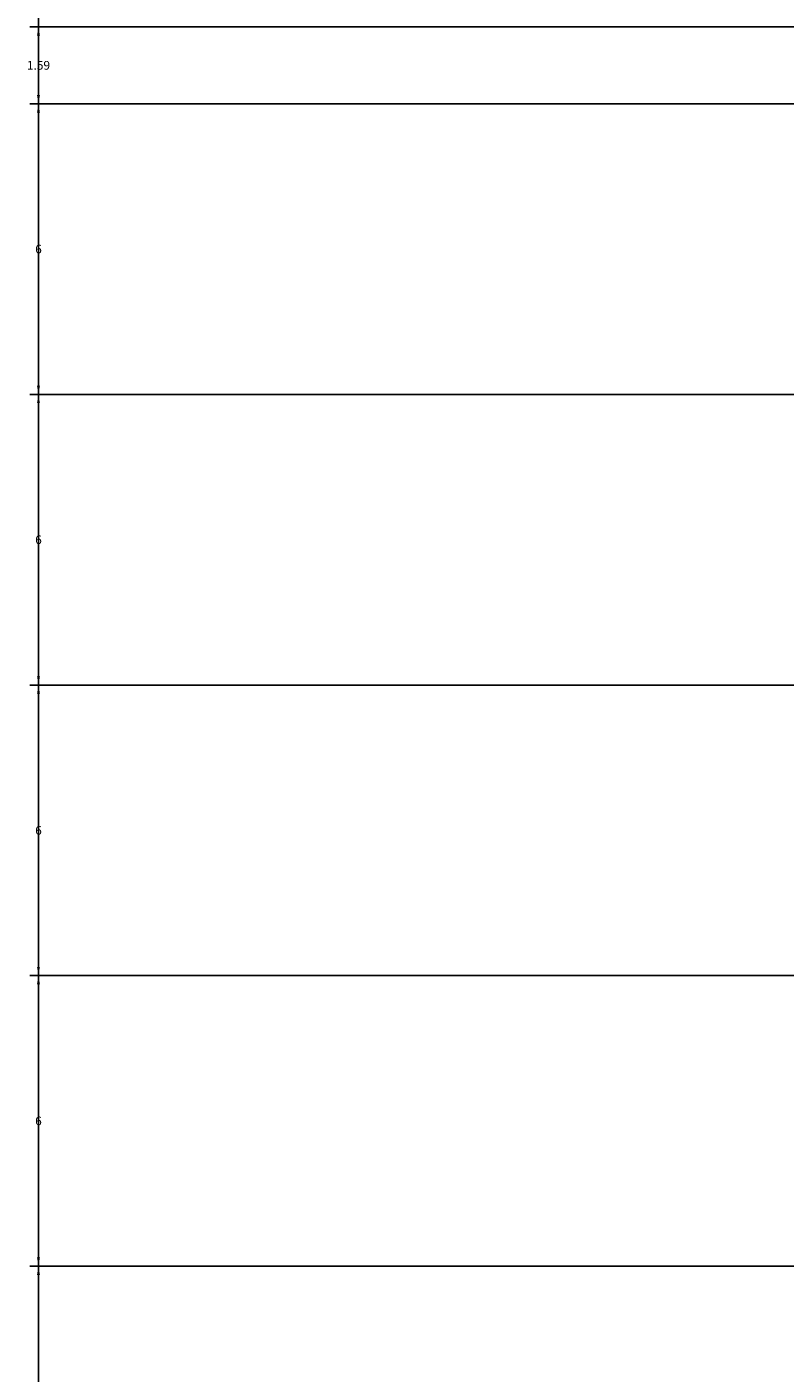
# Model space of a CAD drawing. Units: feet. Extents: x 2695 to 2912, y 795 to 1139.
# Tile 42 of 83: x 2695 to 2710, y 1020 to 1048. Entities that reach past the tile are written whole.
import ezdxf

# ---------------------------------------------------------------- set-up
doc = ezdxf.new("R2010")
doc.units = ezdxf.units.FT
doc.layers.add('A-ANNO-DIMS', color=2, linetype='Continuous', lineweight=18)
doc.styles.get("Standard").update_dxf_attribs({"font": 'arial.ttf'})
doc.dimstyles.get("Standard").update_dxf_attribs({"dimtxt": 0.18, "dimasz": 0.18, "dimexe": 0.18, "dimexo": 0.0625, "dimgap": 0.09, "dimtad": 0, "dimtih": 1, "dimtoh": 1, "dimdec": 1, "dimzin": 0, "dimdsep": 46, "dimlunit": 3, "dimtxsty": 'Standard', "dimcen": 0.09, "dimadec": 0, "dimazin": 0, "dimtfac": 1, "dimtdec": 1, "dimtofl": 0, "dimtmove": 0, "dimatfit": 3, "dimfxl": 1, "dimtolj": 1, "dimtzin": 0, "dimarcsym": 0})

# ---------------------------------------------------------------- blocks, each defined once
blk = doc.blocks.new('*D12')
at = {"layer": 'A-ANNO-DIMS', "color": 0, "lineweight": -2, "transparency": 16777216}
for p, q in [((2710.574, 1122.931), (2694.681, 1122.931)), ((2694.861, 1122.751), (2694.861, 967.113)), ((2694.861, 811.111), (2694.861, 966.749)), ((2710.574, 810.931), (2694.681, 810.931))]:
    blk.add_line(p, q, dxfattribs=at)
at = {"layer": 'A-ANNO-DIMS', "color": 0, "transparency": 16777216}
for points in [[(2694.831, 1122.751), (2694.891, 1122.751), (2694.861, 1122.931)], [(2694.831, 811.111), (2694.891, 811.111), (2694.861, 810.931)]]:
    blk.add_solid(points, dxfattribs=at)
at = {"layer": 'Defpoints', "color": 0, "transparency": 16777216}
for p in [(2694.861, 1122.931), (2710.636, 1122.931), (2710.636, 810.931)]:
    blk.add_point(p, dxfattribs=at)
at = {"layer": 'A-ANNO-DIMS', "color": 0, "transparency": 16777216, "insert": (2694.861, 966.931), "char_height": 0.18, "attachment_point": 5}
blk.add_mtext('\\A1;312', dxfattribs=at)
blk = doc.blocks.new('*D41')
at = {"layer": 'A-ANNO-DIMS', "color": 0, "lineweight": -2, "transparency": 16777216}
for p, q in [((2730.646, 1022.518), (2694.681, 1022.518)), ((2694.861, 1022.338), (2694.861, 1019.7)), ((2694.861, 1016.698), (2694.861, 1019.336)), ((2730.646, 1016.518), (2694.681, 1016.518))]:
    blk.add_line(p, q, dxfattribs=at)
at = {"layer": 'A-ANNO-DIMS', "color": 0, "transparency": 16777216}
for points in [[(2694.831, 1022.338), (2694.891, 1022.338), (2694.861, 1022.518)], [(2694.831, 1016.698), (2694.891, 1016.698), (2694.861, 1016.518)]]:
    blk.add_solid(points, dxfattribs=at)
at = {"layer": 'Defpoints', "color": 0, "transparency": 16777216}
for p in [(2694.861, 1022.518), (2730.708, 1022.518), (2730.708, 1016.518)]:
    blk.add_point(p, dxfattribs=at)
at = {"layer": 'A-ANNO-DIMS', "color": 0, "transparency": 16777216, "insert": (2694.861, 1019.518), "char_height": 0.18, "attachment_point": 5}
blk.add_mtext('\\A1;6', dxfattribs=at)
blk = doc.blocks.new('*D42')
at = {"layer": 'A-ANNO-DIMS', "color": 0, "lineweight": -2, "transparency": 16777216}
for p, q in [((2730.646, 1028.518), (2694.681, 1028.518)), ((2694.861, 1028.338), (2694.861, 1025.7)), ((2694.861, 1022.698), (2694.861, 1025.336)), ((2730.646, 1022.518), (2694.681, 1022.518))]:
    blk.add_line(p, q, dxfattribs=at)
at = {"layer": 'A-ANNO-DIMS', "color": 0, "transparency": 16777216}
for points in [[(2694.831, 1028.338), (2694.891, 1028.338), (2694.861, 1028.518)], [(2694.831, 1022.698), (2694.891, 1022.698), (2694.861, 1022.518)]]:
    blk.add_solid(points, dxfattribs=at)
at = {"layer": 'Defpoints', "color": 0, "transparency": 16777216}
for p in [(2694.861, 1028.518), (2730.708, 1028.518), (2730.708, 1022.518)]:
    blk.add_point(p, dxfattribs=at)
at = {"layer": 'A-ANNO-DIMS', "color": 0, "transparency": 16777216, "insert": (2694.861, 1025.518), "char_height": 0.18, "attachment_point": 5}
blk.add_mtext('\\A1;6', dxfattribs=at)
blk = doc.blocks.new('*D43')
at = {"layer": 'A-ANNO-DIMS', "color": 0, "lineweight": -2, "transparency": 16777216}
for p, q in [((2730.646, 1034.518), (2694.681, 1034.518)), ((2694.861, 1034.338), (2694.861, 1031.7)), ((2694.861, 1028.698), (2694.861, 1031.336)), ((2730.646, 1028.518), (2694.681, 1028.518))]:
    blk.add_line(p, q, dxfattribs=at)
at = {"layer": 'A-ANNO-DIMS', "color": 0, "transparency": 16777216}
for points in [[(2694.831, 1034.338), (2694.891, 1034.338), (2694.861, 1034.518)], [(2694.831, 1028.698), (2694.891, 1028.698), (2694.861, 1028.518)]]:
    blk.add_solid(points, dxfattribs=at)
at = {"layer": 'Defpoints', "color": 0, "transparency": 16777216}
for p in [(2694.861, 1034.518), (2730.708, 1034.518), (2730.708, 1028.518)]:
    blk.add_point(p, dxfattribs=at)
at = {"layer": 'A-ANNO-DIMS', "color": 0, "transparency": 16777216, "insert": (2694.861, 1031.518), "char_height": 0.18, "attachment_point": 5}
blk.add_mtext('\\A1;6', dxfattribs=at)
blk = doc.blocks.new('*D44')
at = {"layer": 'A-ANNO-DIMS', "color": 0, "lineweight": -2, "transparency": 16777216}
for p, q in [((2730.646, 1040.518), (2694.681, 1040.518)), ((2694.861, 1040.338), (2694.861, 1037.7)), ((2694.861, 1034.698), (2694.861, 1037.336)), ((2730.646, 1034.518), (2694.681, 1034.518))]:
    blk.add_line(p, q, dxfattribs=at)
at = {"layer": 'A-ANNO-DIMS', "color": 0, "transparency": 16777216}
for points in [[(2694.831, 1040.338), (2694.891, 1040.338), (2694.861, 1040.518)], [(2694.831, 1034.698), (2694.891, 1034.698), (2694.861, 1034.518)]]:
    blk.add_solid(points, dxfattribs=at)
at = {"layer": 'Defpoints', "color": 0, "transparency": 16777216}
for p in [(2694.861, 1040.518), (2730.708, 1040.518), (2730.708, 1034.518)]:
    blk.add_point(p, dxfattribs=at)
at = {"layer": 'A-ANNO-DIMS', "color": 0, "transparency": 16777216, "insert": (2694.861, 1037.518), "char_height": 0.18, "attachment_point": 5}
blk.add_mtext('\\A1;6', dxfattribs=at)
blk = doc.blocks.new('*D45')
at = {"layer": 'A-ANNO-DIMS', "color": 0, "lineweight": -2, "transparency": 16777216}
for p, q in [((2730.646, 1046.518), (2694.681, 1046.518)), ((2694.861, 1046.338), (2694.861, 1043.7)), ((2694.861, 1040.698), (2694.861, 1043.336)), ((2730.646, 1040.518), (2694.681, 1040.518))]:
    blk.add_line(p, q, dxfattribs=at)
at = {"layer": 'A-ANNO-DIMS', "color": 0, "transparency": 16777216}
for points in [[(2694.831, 1046.338), (2694.891, 1046.338), (2694.861, 1046.518)], [(2694.831, 1040.698), (2694.891, 1040.698), (2694.861, 1040.518)]]:
    blk.add_solid(points, dxfattribs=at)
at = {"layer": 'Defpoints', "color": 0, "transparency": 16777216}
for p in [(2694.861, 1046.518), (2730.708, 1046.518), (2730.708, 1040.518)]:
    blk.add_point(p, dxfattribs=at)
at = {"layer": 'A-ANNO-DIMS', "color": 0, "transparency": 16777216, "insert": (2694.861, 1043.518), "char_height": 0.18, "attachment_point": 5}
blk.add_mtext('\\A1;6', dxfattribs=at)
blk = doc.blocks.new('*D46')
at = {"layer": 'A-ANNO-DIMS', "color": 0, "lineweight": -2, "transparency": 16777216}
for p, q in [((2730.646, 1048.105), (2694.681, 1048.105)), ((2694.861, 1047.925), (2694.861, 1047.493)), ((2694.861, 1046.698), (2694.861, 1047.13)), ((2730.646, 1046.518), (2694.681, 1046.518))]:
    blk.add_line(p, q, dxfattribs=at)
at = {"layer": 'A-ANNO-DIMS', "color": 0, "transparency": 16777216}
for points in [[(2694.831, 1047.925), (2694.891, 1047.925), (2694.861, 1048.105)], [(2694.831, 1046.698), (2694.891, 1046.698), (2694.861, 1046.518)]]:
    blk.add_solid(points, dxfattribs=at)
at = {"layer": 'Defpoints', "color": 0, "transparency": 16777216}
for p in [(2694.861, 1048.105), (2730.708, 1048.105), (2730.708, 1046.518)]:
    blk.add_point(p, dxfattribs=at)
at = {"layer": 'A-ANNO-DIMS', "color": 0, "transparency": 16777216, "insert": (2694.861, 1047.312), "char_height": 0.18, "attachment_point": 5}
blk.add_mtext('\\A1;1.59', dxfattribs=at)

msp = doc.modelspace()

# ---------------------------------------------------------------- dimensions: what is measured, and where the dimension line sits
at = {"layer": 'A-ANNO-DIMS'}
for base, p1, p2, override, picture, middle in [((2694.8611, 1122.9306), (2710.6361, 810.9306), (2710.6361, 1122.9306), {"dimdec": 0, "dimlfac": 1, "dimrnd": 0, "dimzin": 0, "dimdsep": 46, "dimlunit": 2}, '*D12', (2694.8611, 966.9306)), ((2694.8611, 1048.1052), (2730.7081, 1046.5179), (2730.7081, 1048.1052), {"dimdec": 2, "dimlfac": 1, "dimrnd": 0, "dimzin": 0, "dimdsep": 46, "dimlunit": 2}, '*D46', (2694.8611, 1047.3116)), ((2694.8611, 1046.5179), (2730.7081, 1040.5179), (2730.7081, 1046.5179), {"dimdec": 0, "dimlfac": 1, "dimrnd": 0, "dimzin": 0, "dimdsep": 46, "dimlunit": 2}, '*D45', (2694.8611, 1043.5179)), ((2694.8611, 1040.5179), (2730.7081, 1034.5179), (2730.7081, 1040.5179), {"dimdec": 0, "dimlfac": 1, "dimrnd": 0, "dimzin": 0, "dimdsep": 46, "dimlunit": 2}, '*D44', (2694.8611, 1037.5179)), ((2694.8611, 1034.5179), (2730.7081, 1028.5179), (2730.7081, 1034.5179), {"dimdec": 0, "dimlfac": 1, "dimrnd": 0, "dimzin": 0, "dimdsep": 46, "dimlunit": 2}, '*D43', (2694.8611, 1031.5179)), ((2694.8611, 1028.5179), (2730.7081, 1022.5179), (2730.7081, 1028.5179), {"dimdec": 0, "dimlfac": 1, "dimrnd": 0, "dimzin": 0, "dimdsep": 46, "dimlunit": 2}, '*D42', (2694.8611, 1025.5179)), ((2694.8611, 1022.5179), (2730.7081, 1016.5179), (2730.7081, 1022.5179), {"dimdec": 0, "dimlfac": 1, "dimrnd": 0, "dimzin": 0, "dimdsep": 46, "dimlunit": 2}, '*D41', (2694.8611, 1019.5179))]:
    dim = msp.add_linear_dim(base=base, p1=p1, p2=p2, angle=90, dimstyle='Standard', override=override, dxfattribs=at)
    dim.commit()
    dim.dimension.update_dxf_attribs({"geometry": picture, "text_midpoint": middle})

doc.saveas('drawing.dxf')
